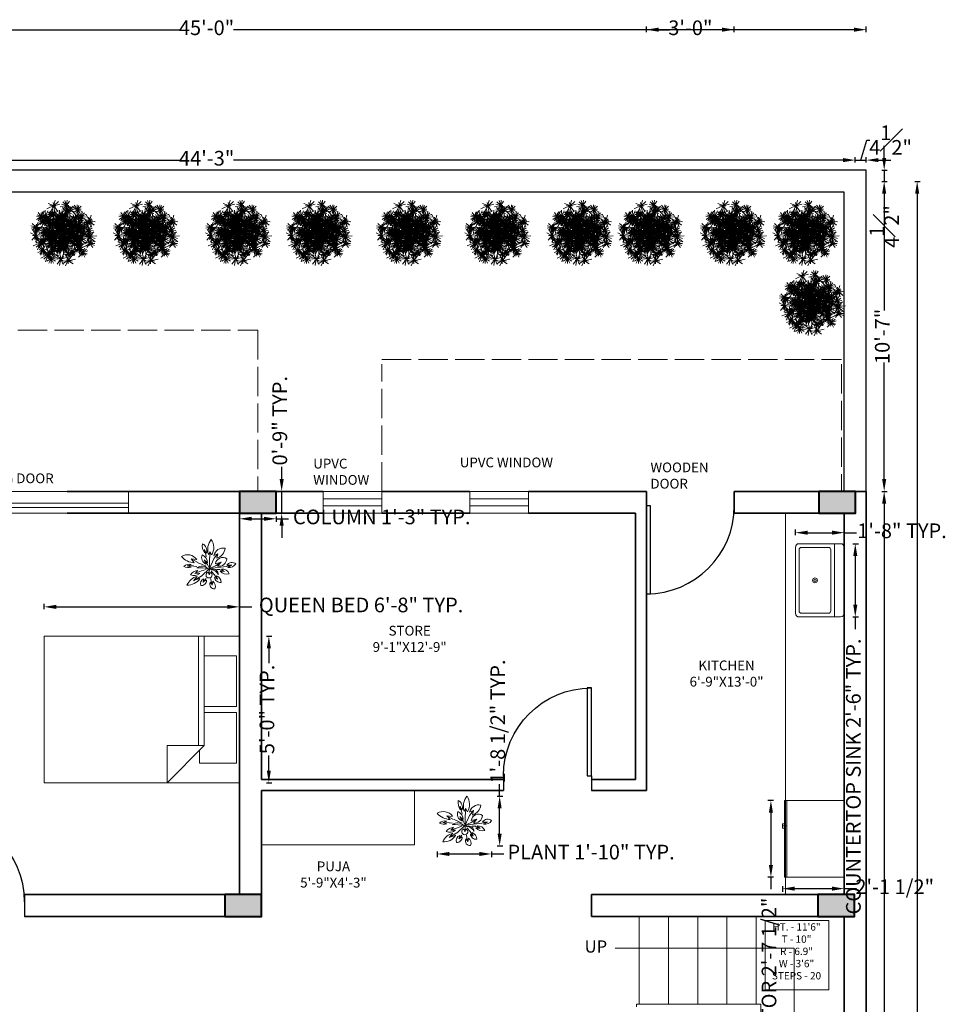
# Model space of a CAD drawing. Units: inches. Extents: x 2845 to 3575, y 808 to 1996.
# Tile 6 of 6: x 3166 to 3545, y 1588 to 1991. Entities that reach past the tile are written whole.
import ezdxf

# ---------------------------------------------------------------- set-up
doc = ezdxf.new("R2010")
doc.units = ezdxf.units.IN
doc.linetypes.add('ACAD_ISO02W100', pattern=[15, 12, -3])
for name, color, linetype, lineweight in [('A-ANNO-DIMS', 2, 'Continuous', 18), ('A-ANNO-SYMB', 7, 'Continuous', 18), ('A-ANNO-TEXT', 7, 'Continuous', 18), ('A-AREA-IDEN', 7, 'Continuous', 18), ('A-COLS', 7, 'Continuous', 40), ('A-DOOR', 34, 'Continuous', 25), ('A-EQPM', 8, 'Continuous', 18), ('A-FLOR-CASE', 30, 'Continuous', 18), ('A-FLOR-FIXT', 8, 'Continuous', 18), ('A-FLOR-STRS', 142, 'Continuous', 18), ('A-FURN', 30, 'Continuous', 18), ('A-GLAZ', 4, 'Continuous', 18), ('A-ROOF-OVHD', 7, 'ACAD_ISO02W100', 18), ('A-WALL', 1, 'Continuous', 35), ('C-PROP', 7, 'Continuous', 30), ('L-PLNT', 3, 'Continuous', 13)]:
    doc.layers.add(name, color=color, linetype=linetype, lineweight=lineweight)
doc.styles.get("Standard").update_dxf_attribs({"font": 'arial.ttf'})
doc.dimstyles.new('ISO-25', dxfattribs={"dimtxt": 6, "dimasz": 5, "dimexe": 1.25, "dimexo": 0.625, "dimtad": 0, "dimlunit": 4, "dimtxsty": 'Standard', "dimcen": 2.5, "dimclrd": 1, "dimclre": 1, "dimclrt": 1, "dimadec": 0, "dimazin": 0, "dimtfac": 1, "dimtmove": 0, "dimatfit": 3, "dimfxl": 1, "dimfxlon": 1, "dimfrac": 1, "dimarcsym": 0})

# ---------------------------------------------------------------- blocks, each defined once
blk = doc.blocks.new('*U3')
for p, q in [((0, 0), (0, -6)), ((36, 0), (36, -6))]:
    blk.add_line(p, q)
blk.add_lwpolyline([(0, 0), (0, 36), (1.75, 36), (1.75, 0)], close=True)
blk.add_arc((0, 0), 36, 0, 90)
blk = doc.blocks.new('*U7')
for p, q in [((0, 0), (0, 6)), ((36, 0), (36, 6))]:
    blk.add_line(p, q)
blk.add_lwpolyline([(0, 0), (0, -36), (1.75, -36), (1.75, 0)], close=True)
blk.add_arc((0, 0), 36, 270, 0)
blk = doc.blocks.new('Bed - Queen')
for p, q in [((0, -80.00003), (0, 0)), ((0, 0), (59.99999, 0)), ((59.99999, 0), (59.99999, -80.00003)), ((7.99999, -1.2), (28.79998, -1.2)), ((7.99999, -14.4), (7.99999, -1.2)), ((28.79998, -1.2), (28.79998, -14.4)), ((31.19999, -1.2), (51.99999, -1.2)), ((31.19999, -14.4), (31.19999, -1.2)), ((51.99999, -1.2), (51.99999, -16.4)), ((0, -14.4), (44.8, -14.4)), ((59.99999, -29.6), (44.8, -14.4)), ((44.8, -14.4), (44.8, -29.6)), ((44.8, -16.8), (0, -16.8)), ((51.99999, -16.4), (46.79936, -16.4)), ((44.8, -29.6), (59.99999, -29.6)), ((59.99999, -80.00003), (0, -80.00003))]:
    blk.add_line(p, q)
blk = doc.blocks.new('Sink-single - 30 in top')
blk.add_line((-15, -3.999996), (15, -3.999996))
for points in [[(-13.5, 0), (13.5, 0)], [(-15, -18.499996), (-15, -1.5)], [(15, -1.5), (15, -18.499996)], [(-13.5, -17.499996), (-13.5, -6.499996)], [(-12.5, -5.499996), (12.5, -5.499996)], [(13.5, -6.499996), (13.5, -17.499996)], [(13.5, -19.999996), (-13.5, -19.999996)], [(12.5, -18.499996), (-12.5, -18.499996)]]:
    blk.add_lwpolyline(points)
for radius in [1, 0.5]:
    blk.add_circle((0, -11.999996), radius)
for centre, radius, start, end in [((-13.5, -1.5), 1.5, 90, 180), ((13.5, -1.5), 1.5, 0, 90), ((-12.5, -6.499996), 1, 90, 180), ((12.5, -6.499996), 1, 0, 90), ((-13.5, -18.499996), 1.5, 180, 270), ((-12.5, -17.499996), 1, 180, 270), ((12.5, -17.499996), 1, 270, 0), ((13.5, -18.499996), 1.5, 270, 0)]:
    blk.add_arc(centre, radius, start, end)
blk = doc.blocks.new('Refrigerator-2 door - 36 in top')
for p, q in [((0, -26.999999), (36, -26.999999)), ((12, -26.999999), (12, -28.999999)), ((11, -27.999999), (11, -28.999999)), ((11, -28.999999), (13, -28.999999)), ((13, -28.999999), (13, -27.999999))]:
    blk.add_line(p, q)
blk.add_lwpolyline([(0, -27.999999), (0, 0), (36, 0), (36, -27.999999)], close=True)
blk = doc.blocks.new('z_96')
for p, q in [((-282, 143), (-440, 264)), ((-279, 140), (-327, 271)), ((-280, 150), (-254, 304)), ((-277, 144), (-209, 319)), ((2, 182), (-93, 262)), ((-2, 184), (-55, 292)), ((1, 182), (29, 300)), ((4, 189), (59, 265)), ((6, 185), (92, 285)), ((-283, 139), (-471, 115)), ((-292, 134), (-431, 180)), ((-279, 142), (-398, 17)), ((-286, 137), (-375, 92)), ((-278, 140), (-313, -1)), ((-279, 135), (-307, 100)), ((-280, 150), (-304, 174)), ((-278, 131), (-222, 40)), ((-277, 137), (-129, 19)), ((-276, 141), (-147, 221)), ((-18, -6), (-275, 142)), ((-263, 140), (-131, 114)), ((-260, 142), (-98, 156)), ((-10, 183), (-130, 223)), ((-75, -25), (-112, 38)), ((-6, 186), (-100, 114)), ((-5, 182), (-87, 72)), ((-72, -35), (-42, 65)), ((-5, -3), (1, 176)), ((-1, 185), (126, 194)), ((0, 0), (389, 84)), ((2, 183), (70, 78)), ((10, 182), (88, 115)), ((164, -90), (143, 12)), ((163, -89), (239, 8)), ((393, 90), (274, 50)), ((393, 90), (285, 153)), ((393, 90), (294, 12)), ((393, 90), (354, 209)), ((391, 83), (363, 42)), ((393, 90), (479, 182)), ((393, 90), (515, 124)), ((393, 90), (494, 13)), ((393, 90), (517, 64)), ((393, 90), (443, -26)), ((396, 95), (439, 246)), ((409, 93), (456, 89)), ((-237, -199), (-392, -169)), ((-242, -196), (-391, -241)), ((-242, -199), (-330, -310)), ((-246, -194), (-283, -164)), ((-237, -199), (-267, -22)), ((-241, -202), (-259, -277)), ((-242, -202), (-48, -207)), ((-10, -6), (-236, -205)), ((-236, -201), (-139, -307)), ((-234, -202), (-196, -41)), ((-231, -196), (-205, -162)), ((-231, -206), (-147, -236)), ((-75, -39), (-157, -75)), ((-74, -33), (-152, -41)), ((-65, -33), (-136, -11)), ((-76, -36), (-103, -106)), ((-80, -29), (-90, -20)), ((-16, -6), (-75, -37)), ((-73, -35), (-72, -112)), ((-70, -40), (-38, -103)), ((-70, -41), (4, -57)), ((-68, -28), (-56, -19)), ((-5, -19), (164, -92)), ((167, -95), (37, -175)), ((161, -92), (74, -95)), ((159, -86), (86, -29)), ((164, -102), (119, -171)), ((163, -86), (138, -56)), ((164, -93), (157, -141)), ((160, -93), (268, -148)), ((164, -92), (234, -170)), ((165, -92), (296, -74)), ((167, -88), (276, -25)), ((167, -91), (187, -100)), ((167, -104), (188, -213)), ((168, -88), (194, -72))]:
    blk.add_line(p, q)
blk = doc.blocks.new('сосна 1')
for p, rotation in [((318, 388), 121.1570021628385), ((-413, 387), 205.4822314301707), ((-343, -102), 57.88453704712605), ((-351, 122), 257.3134436407499), ((-143, -5), 121.1570021628385), ((-137, 361), 177.7388340989747), ((-117, 122), 55.05972244949475), ((286, 9), 60.73020616460848), ((234, -65), 73.8676290404427), ((-274, 161), 177.7388340989747), ((98, -5), 177.7388340989747), ((174, 17), 349.7944254651076), ((327, 46), 177.7388340989747), ((-502, -282), 279.7984529833926), ((-175, -367), 63.19571700542104), ((-49, -394), 342.5348703671633), ((261, -459), 13.72293452966709)]:
    blk.add_blockref('z_96', p, dxfattribs=dict(rotation=rotation))
blk = doc.blocks.new('z_109')
for p, q in [((-392, 202), (-278, 190)), ((-254, 128), (-392, 202)), ((-390, 202), (-327, 125)), ((-94, 294), (-122, 396)), ((-121, 393), (-119, 324)), ((-120, 377), (-82, 322)), ((-85, 244), (-94, 293)), ((-5, 350), (-42, 295)), ((-20, 11), (-18, 230)), ((-20, 11), (65, 205)), ((-14, 234), (-5, 350)), ((-5, 350), (24, 284)), ((65, 209), (150, 307)), ((65, 205), (65, 205)), ((150, 307), (68, 272)), ((129, 216), (150, 307)), ((150, 307), (129, 216)), ((-342, 60), (-472, 63)), ((-467, 63), (-392, 90)), ((-463, 64), (-392, 37)), ((-276, 53), (-338, 57)), ((-84, 54), (-246, 125)), ((-20, 11), (-181, -143)), ((-61, 92), (-128, 186)), ((-126, 184), (-60, 125)), ((-120, 176), (-91, 98)), ((-20, 11), (-61, 92)), ((-20, 11), (-24, -65)), ((-20, 11), (102, 64)), ((-20, 11), (-14, 11)), ((-14, 11), (319, 50)), ((-14, 11), (-13, 13)), ((-13, 13), (13, -13)), ((217, 135), (101, 105)), ((102, 64), (217, 135)), ((217, 135), (145, 55)), ((319, 50), (434, 75)), ((429, 74), (333, 77)), ((428, 74), (353, 32)), ((-187, -143), (-345, -240)), ((-342, -238), (-269, -151)), ((-328, -230), (-213, -195)), ((-178, -41), (-313, -92)), ((-308, -90), (-254, -33)), ((-306, -89), (-217, -88)), ((-86, -8), (-178, -41)), ((-89, -192), (-150, -267)), ((-150, -266), (-131, -199)), ((-26, -113), (-45, -66)), ((-24, -65), (-28, -121)), ((-28, -117), (-2, -69)), ((4, -192), (16, -238)), ((16, -43), (88, -126)), ((141, -208), (84, -170)), ((87, -129), (140, -204)), ((122, -8), (193, -11)), ((140, -205), (123, -139)), ((176, -10), (285, -54)), ((283, -54), (196, -42)), ((273, -52), (222, -4)), ((-151, -267), (-81, -228)), ((34, -320), (-6, -268)), ((16, -238), (35, -326)), ((35, -327), (45, -249))]:
    blk.add_line(p, q)
for centre, radius, start, end in [((84, 468), 249, 170.3029, 215.3262), ((-235, 368), 160, 343.2534, 62.5239), ((262, 393), 319, 140.563, 197.8988), ((-221, 433), 288, 328.6458, 34.5329), ((256, 231), 192, 77.7318, 167.6805), ((55, 447), 242, 287.7269, 353.3689), ((-464, 59), 228, 35.1725, 122.5976), ((-304, 504), 380, 221.8384, 266.6027), ((-21, 239), 158, 161.4501, 243.415), ((-251, 115), 192, 2.9136, 65.0019), ((247, 86), 147, 55.2824, 172.6291), ((167, 217), 164, 262.2896, 356.2544), ((-434, -39), 136, 71.6414, 139.5892), ((-450, 225), 197, 243.5199, 287.2599), ((-173, -118), 175, 44.3837, 127.1057), ((-243, -1063), 1086, 79.6239, 91.8656), ((434, 8), 123, 51.1111, 145.9654), ((384, 175), 146, 257.8549, 330.7421), ((-198, -444), 302, 103.499, 156.8265), ((-455, -39), 287, 265.8156, 327.2626), ((-246, -222), 190, 92.4489, 147.0817), ((-337, 52), 185, 248.0932, 310.529), ((-94, -301), 109, 109.8936, 199.3062), ((-31, -123), 58.9, 103.4106, 268.148), ((-26, -123), 58.9, 262.5922, 66.6581), ((53, -110), 105, 354.7987, 111.9005), ((2, -181), 167, 21.6922, 85.2277), ((197, -160), 113, 185.1842, 278.9266), ((66, -276), 148, 1.4924, 67.3596), ((325, 60), 164, 218.6232, 288.4099), ((241, -149), 146, 21.4559, 97.3107), ((-186, -232), 105, 264.4232, 2.0221), ((80, -308), 95.1, 155.1092, 275.9038), ((-28, -354), 128, 337.3115, 55.0978)]:
    blk.add_arc(centre, radius, start, end)
blk = doc.blocks.new('*D23')
at = {"layer": 'A-ANNO-DIMS', "color": 0, "lineweight": -2, "transparency": 16777216}
for p, q in [((2977.22, 1932.77), (2977.22, 1935.02)), ((3508.12, 1932.77), (3508.12, 1935.02)), ((2982.22, 1933.77), (3231.61, 1933.77)), ((3503.12, 1933.77), (3253.72, 1933.77))]:
    blk.add_line(p, q, dxfattribs=at)
at = {"layer": 'A-ANNO-DIMS', "color": 0, "transparency": 16777216}
for points in [[(2982.22, 1934.61), (2982.22, 1932.94), (2977.22, 1933.77)], [(3503.12, 1934.61), (3503.12, 1932.94), (3508.12, 1933.77)]]:
    blk.add_solid(points, dxfattribs=at)
at = {"layer": 'Defpoints', "color": 0, "transparency": 16777216}
for p in [(3508.12, 1933.77), (2977.22, 1929.67), (3508.12, 1920.75)]:
    blk.add_point(p, dxfattribs=at)
at = {"layer": 'A-ANNO-DIMS', "color": 0, "transparency": 16777216, "insert": (3242.67, 1933.77), "char_height": 6, "attachment_point": 5}
blk.add_mtext('44\'-3"', dxfattribs=at)
blk = doc.blocks.new('*D24')
at = {"layer": 'A-ANNO-DIMS', "color": 0, "lineweight": -2, "transparency": 16777216}
for p, q in [((3510.37, 1933.77), (3512.83, 1941.99)), ((3512.83, 1941.99), (3514.08, 1941.99)), ((3508.12, 1932.77), (3508.12, 1935.02)), ((3512.62, 1932.77), (3512.62, 1935.02)), ((3503.12, 1933.77), (3498.12, 1933.77)), ((3508.12, 1933.77), (3512.62, 1933.77)), ((3508.12, 1933.77), (3512.62, 1933.77)), ((3517.62, 1933.77), (3522.62, 1933.77))]:
    blk.add_line(p, q, dxfattribs=at)
at = {"layer": 'A-ANNO-DIMS', "color": 0, "transparency": 16777216}
for points in [[(3503.12, 1934.61), (3503.12, 1932.94), (3508.12, 1933.77)], [(3517.62, 1934.61), (3517.62, 1932.94), (3512.62, 1933.77)]]:
    blk.add_solid(points, dxfattribs=at)
at = {"layer": 'Defpoints', "color": 0, "transparency": 16777216}
for p in [(3512.62, 1933.77), (3512.62, 1929.67), (3508.12, 1920.75)]:
    blk.add_point(p, dxfattribs=at)
at = {"layer": 'A-ANNO-DIMS', "color": 0, "transparency": 16777216, "insert": (3522.57, 1941.99), "char_height": 6, "attachment_point": 5}
blk.add_mtext('4{\\H1x;\\S1#2;}"', dxfattribs=at)
blk = doc.blocks.new('*D25')
at = {"layer": 'A-ANNO-DIMS', "color": 0, "lineweight": -2, "transparency": 16777216}
for p, q in [((3519.95, 1934.67), (3519.95, 1939.67)), ((3518.95, 1929.67), (3521.2, 1929.67)), ((3519.95, 1929.67), (3519.95, 1925.07)), ((3518.95, 1925.07), (3521.2, 1925.07)), ((3519.95, 1920.07), (3519.95, 1915.07))]:
    blk.add_line(p, q, dxfattribs=at)
at = {"layer": 'A-ANNO-DIMS', "color": 0, "transparency": 16777216}
for points in [[(3519.11, 1934.67), (3520.78, 1934.67), (3519.95, 1929.67)], [(3519.11, 1920.07), (3520.78, 1920.07), (3519.95, 1925.07)]]:
    blk.add_solid(points, dxfattribs=at)
at = {"layer": 'Defpoints', "color": 0, "transparency": 16777216}
for p in [(3512.62, 1929.67), (3512.62, 1925.07), (3519.95, 1925.07)]:
    blk.add_point(p, dxfattribs=at)
at = {"layer": 'A-ANNO-DIMS', "color": 0, "transparency": 16777216, "insert": (3519.95, 1906.59), "char_height": 6, "attachment_point": 5, "rotation": 90}
blk.add_mtext('4{\\H1x;\\S1#2;}"', dxfattribs=at)
blk = doc.blocks.new('*D26')
at = {"layer": 'A-ANNO-DIMS', "color": 0, "lineweight": -2, "transparency": 16777216}
for p, q in [((3518.95, 1925.07), (3521.2, 1925.07)), ((3519.95, 1920.07), (3519.95, 1872.27)), ((3519.95, 1803.17), (3519.95, 1850.97)), ((3518.95, 1798.17), (3521.2, 1798.17))]:
    blk.add_line(p, q, dxfattribs=at)
at = {"layer": 'A-ANNO-DIMS', "color": 0, "transparency": 16777216}
for points in [[(3519.11, 1920.07), (3520.78, 1920.07), (3519.95, 1925.07)], [(3519.11, 1803.17), (3520.78, 1803.17), (3519.95, 1798.17)]]:
    blk.add_solid(points, dxfattribs=at)
at = {"layer": 'Defpoints', "color": 0, "transparency": 16777216}
for p in [(3512.62, 1925.07), (3512.62, 1798.17), (3519.95, 1798.17)]:
    blk.add_point(p, dxfattribs=at)
at = {"layer": 'A-ANNO-DIMS', "color": 0, "transparency": 16777216, "insert": (3519.95, 1861.62), "char_height": 6, "attachment_point": 5, "rotation": 90}
blk.add_mtext('10\'-7"', dxfattribs=at)
blk = doc.blocks.new('*D27')
at = {"layer": 'A-ANNO-DIMS', "color": 0, "lineweight": -2, "transparency": 16777216}
for p, q in [((3518.95, 1798.17), (3521.2, 1798.17)), ((3519.95, 1793.17), (3519.95, 1512.51)), ((3519.95, 1220.17), (3519.95, 1500.84)), ((3518.95, 1215.17), (3521.2, 1215.17))]:
    blk.add_line(p, q, dxfattribs=at)
at = {"layer": 'A-ANNO-DIMS', "color": 0, "transparency": 16777216}
for points in [[(3519.11, 1793.17), (3520.78, 1793.17), (3519.95, 1798.17)], [(3519.11, 1220.17), (3520.78, 1220.17), (3519.95, 1215.17)]]:
    blk.add_solid(points, dxfattribs=at)
at = {"layer": 'Defpoints', "color": 0, "transparency": 16777216}
for p in [(3512.62, 1798.17), (3507.65, 1215.17), (3519.95, 1215.17)]:
    blk.add_point(p, dxfattribs=at)
at = {"layer": 'A-ANNO-DIMS', "color": 0, "transparency": 16777216, "insert": (3519.95, 1506.67), "char_height": 6, "attachment_point": 5, "rotation": 90}
blk.add_mtext("49'", dxfattribs=at)
blk = doc.blocks.new('*D29')
at = {"layer": 'A-ANNO-DIMS', "color": 0, "lineweight": -2, "transparency": 16777216}
for p, q in [((3532.44, 1925.07), (3534.69, 1925.07)), ((3533.44, 1920.07), (3533.44, 1464.53)), ((3533.44, 987.17), (3533.44, 1442.72)), ((3532.44, 982.17), (3534.69, 982.17))]:
    blk.add_line(p, q, dxfattribs=at)
at = {"layer": 'A-ANNO-DIMS', "color": 0, "transparency": 16777216}
for points in [[(3532.6, 1920.07), (3534.27, 1920.07), (3533.44, 1925.07)], [(3532.6, 987.17), (3534.27, 987.17), (3533.44, 982.17)]]:
    blk.add_solid(points, dxfattribs=at)
at = {"layer": 'Defpoints', "color": 0, "transparency": 16777216}
for p in [(3519.95, 1925.07), (3533.44, 1925.07), (3512.62, 982.17)]:
    blk.add_point(p, dxfattribs=at)
at = {"layer": 'A-ANNO-DIMS', "color": 0, "transparency": 16777216, "insert": (3533.44, 1453.62), "char_height": 6, "attachment_point": 5, "rotation": 90}
blk.add_mtext('78\'-7"', dxfattribs=at)
blk = doc.blocks.new('COL-15x9')
h = blk.add_hatch(color=256)
h.dxf.hatch_style = 1
h.paths.add_polyline_path([(15, 9), (0, 9), (0, 0), (15, 0)])
blk.add_lwpolyline([(0, 9), (0, 0), (15, 0), (15, 9)], close=True)
blk = doc.blocks.new('WIN-24')
for p, q in [((0, 9), (0, 0)), ((0, 9), (24, 9)), ((24, 9), (24, 0)), ((0, 6), (24, 6)), ((0, 3), (24, 3)), ((0, 0), (24, 0))]:
    blk.add_line(p, q)
blk = doc.blocks.new('GLAZ-SLIDER-97')
for p, q in [((0, 9), (0, 0)), ((0, 9), (97.12, 9)), ((97.12, 9), (97.12, 0)), ((0, 6.63), (48.56, 6.63)), ((48.56, 4.89), (0, 4.89)), ((48.56, 6.63), (48.56, 4.89)), ((48.56, 2.45), (48.56, 4.19)), ((48.56, 4.19), (97.12, 4.19)), ((0, 0), (97.12, 0)), ((97.12, 2.45), (48.56, 2.45))]:
    blk.add_line(p, q)
blk = doc.blocks.new('*D40')
at = {"layer": 'A-ANNO-DIMS', "color": 1, "lineweight": -2, "transparency": 16777216}
for p, q in [((3337.01, 1650.72), (3337.01, 1648.47)), ((3342.01, 1649.72), (3354.24, 1649.72)), ((3359.24, 1650.72), (3359.24, 1648.47)), ((3359.24, 1649.72), (3364.24, 1649.72))]:
    blk.add_line(p, q, dxfattribs=at)
at = {"layer": 'A-ANNO-DIMS', "color": 1, "transparency": 16777216}
for points in [[(3342.01, 1650.55), (3342.01, 1648.89), (3337.01, 1649.72)], [(3354.24, 1650.55), (3354.24, 1648.89), (3359.24, 1649.72)]]:
    blk.add_solid(points, dxfattribs=at)
at = {"layer": 'Defpoints', "color": 0, "transparency": 16777216}
for p in [(3337.01, 1653.05), (3359.24, 1653.05), (3359.24, 1649.72)]:
    blk.add_point(p, dxfattribs=at)
at = {"layer": 'A-ANNO-DIMS', "color": 1, "transparency": 16777216, "insert": (3400, 1649.72), "char_height": 6, "attachment_point": 5}
blk.add_mtext('PLANT 1\'-10" TYP.', dxfattribs=at)
blk = doc.blocks.new('*D41')
at = {"layer": 'A-ANNO-DIMS', "color": 1, "lineweight": -2, "transparency": 16777216}
for p, q in [((3362.57, 1673.34), (3362.57, 1678.34)), ((3361.57, 1673.34), (3363.82, 1673.34)), ((3362.57, 1658.05), (3362.57, 1668.34)), ((3361.57, 1653.05), (3363.82, 1653.05))]:
    blk.add_line(p, q, dxfattribs=at)
at = {"layer": 'A-ANNO-DIMS', "color": 1, "transparency": 16777216}
for points in [[(3361.74, 1668.34), (3363.4, 1668.34), (3362.57, 1673.34)], [(3361.74, 1658.05), (3363.4, 1658.05), (3362.57, 1653.05)]]:
    blk.add_solid(points, dxfattribs=at)
at = {"layer": 'Defpoints', "color": 0, "transparency": 16777216}
for p in [(3359.24, 1673.34), (3362.57, 1673.34), (3359.24, 1653.05)]:
    blk.add_point(p, dxfattribs=at)
at = {"layer": 'A-ANNO-DIMS', "color": 1, "transparency": 16777216, "insert": (3362.57, 1703.96), "char_height": 6, "attachment_point": 5, "rotation": 90}
blk.add_mtext('1\'-8 1/2" TYP.', dxfattribs=at)
blk = doc.blocks.new('*D42')
at = {"layer": 'A-ANNO-DIMS', "color": 1, "lineweight": -2, "transparency": 16777216}
for p, q in [((3256.12, 1787.92), (3256.12, 1785.67)), ((3261.12, 1786.92), (3266.12, 1786.92)), ((3271.12, 1787.92), (3271.12, 1785.67)), ((3271.12, 1786.92), (3276.12, 1786.92))]:
    blk.add_line(p, q, dxfattribs=at)
at = {"layer": 'A-ANNO-DIMS', "color": 1, "transparency": 16777216}
for points in [[(3261.12, 1787.76), (3261.12, 1786.09), (3256.12, 1786.92)], [(3266.12, 1787.76), (3266.12, 1786.09), (3271.12, 1786.92)]]:
    blk.add_solid(points, dxfattribs=at)
at = {"layer": 'Defpoints', "color": 0, "transparency": 16777216}
for p in [(3256.12, 1789.17), (3271.12, 1789.17), (3271.12, 1786.92)]:
    blk.add_point(p, dxfattribs=at)
at = {"layer": 'A-ANNO-DIMS', "color": 1, "transparency": 16777216, "insert": (3314.32, 1786.92), "char_height": 6, "attachment_point": 5}
blk.add_mtext('COLUMN 1\'-3" TYP.', dxfattribs=at)
blk = doc.blocks.new('*D43')
at = {"layer": 'A-ANNO-DIMS', "color": 1, "lineweight": -2, "transparency": 16777216}
for p, q in [((3273.37, 1803.17), (3273.37, 1808.17)), ((3272.37, 1798.17), (3274.62, 1798.17)), ((3273.37, 1789.17), (3273.37, 1798.17)), ((3272.37, 1789.17), (3274.62, 1789.17)), ((3273.37, 1784.17), (3273.37, 1779.17))]:
    blk.add_line(p, q, dxfattribs=at)
at = {"layer": 'A-ANNO-DIMS', "color": 1, "transparency": 16777216}
for points in [[(3272.53, 1803.17), (3274.2, 1803.17), (3273.37, 1798.17)], [(3272.53, 1784.17), (3274.2, 1784.17), (3273.37, 1789.17)]]:
    blk.add_solid(points, dxfattribs=at)
at = {"layer": 'Defpoints', "color": 0, "transparency": 16777216}
for p in [(3271.12, 1798.17), (3273.37, 1798.17), (3271.12, 1789.17)]:
    blk.add_point(p, dxfattribs=at)
at = {"layer": 'A-ANNO-DIMS', "color": 1, "transparency": 16777216, "insert": (3273.37, 1827.08), "char_height": 6, "attachment_point": 5, "rotation": 90}
blk.add_mtext('0\'-9" TYP.', dxfattribs=at)
blk = doc.blocks.new('*D48')
at = {"layer": 'A-ANNO-DIMS', "color": 1, "lineweight": -2, "transparency": 16777216}
for p, q in [((3507.12, 1776.75), (3509.37, 1776.75)), ((3508.12, 1771.75), (3508.12, 1751.75)), ((3507.12, 1746.75), (3509.37, 1746.75)), ((3508.12, 1746.75), (3508.12, 1741.75))]:
    blk.add_line(p, q, dxfattribs=at)
at = {"layer": 'A-ANNO-DIMS', "color": 1, "transparency": 16777216}
for points in [[(3507.28, 1771.75), (3508.95, 1771.75), (3508.12, 1776.75)], [(3507.28, 1751.75), (3508.95, 1751.75), (3508.12, 1746.75)]]:
    blk.add_solid(points, dxfattribs=at)
at = {"layer": 'Defpoints', "color": 0, "transparency": 16777216}
for p in [(3503.62, 1776.75), (3503.62, 1746.75), (3508.12, 1746.75)]:
    blk.add_point(p, dxfattribs=at)
at = {"layer": 'A-ANNO-DIMS', "color": 1, "transparency": 16777216, "insert": (3508.12, 1681.43), "char_height": 6, "attachment_point": 5, "rotation": 90}
blk.add_mtext('COUNTERTOP SINK 2\'-6" TYP.', dxfattribs=at)
blk = doc.blocks.new('*D49')
at = {"layer": 'A-ANNO-DIMS', "color": 1, "lineweight": -2, "transparency": 16777216}
for p, q in [((3483.62, 1780.25), (3483.62, 1782.5)), ((3503.62, 1780.25), (3503.62, 1782.5)), ((3488.62, 1781.25), (3498.62, 1781.25)), ((3503.62, 1781.25), (3508.62, 1781.25))]:
    blk.add_line(p, q, dxfattribs=at)
at = {"layer": 'A-ANNO-DIMS', "color": 1, "transparency": 16777216}
for points in [[(3488.62, 1782.08), (3488.62, 1780.42), (3483.62, 1781.25)], [(3498.62, 1782.08), (3498.62, 1780.42), (3503.62, 1781.25)]]:
    blk.add_solid(points, dxfattribs=at)
at = {"layer": 'Defpoints', "color": 0, "transparency": 16777216}
for p in [(3503.62, 1781.25), (3483.62, 1776.75), (3503.62, 1776.75)]:
    blk.add_point(p, dxfattribs=at)
at = {"layer": 'A-ANNO-DIMS', "color": 1, "transparency": 16777216, "insert": (3527.24, 1781.25), "char_height": 6, "attachment_point": 5}
blk.add_mtext('1\'-8" TYP.', dxfattribs=at)
blk = doc.blocks.new('*D50')
at = {"layer": 'A-ANNO-DIMS', "color": 1, "lineweight": -2, "transparency": 16777216}
for p, q in [((3176.12, 1749.88), (3176.12, 1752.13)), ((3181.12, 1750.88), (3251.12, 1750.88)), ((3256.12, 1749.88), (3256.12, 1752.13)), ((3256.12, 1750.88), (3261.12, 1750.88))]:
    blk.add_line(p, q, dxfattribs=at)
at = {"layer": 'A-ANNO-DIMS', "color": 1, "transparency": 16777216}
for points in [[(3181.12, 1751.71), (3181.12, 1750.04), (3176.12, 1750.88)], [(3251.12, 1751.71), (3251.12, 1750.04), (3256.12, 1750.88)]]:
    blk.add_solid(points, dxfattribs=at)
at = {"layer": 'Defpoints', "color": 0, "transparency": 16777216}
for p in [(3256.12, 1750.88), (3176.12, 1738.88), (3256.12, 1738.88)]:
    blk.add_point(p, dxfattribs=at)
at = {"layer": 'A-ANNO-DIMS', "color": 1, "transparency": 16777216, "insert": (3305.87, 1750.88), "char_height": 6, "attachment_point": 5}
blk.add_mtext('QUEEN BED 6\'-8" TYP.', dxfattribs=at)
blk = doc.blocks.new('*D51')
at = {"layer": 'A-ANNO-DIMS', "color": 1, "lineweight": -2, "transparency": 16777216}
for p, q in [((3267.12, 1738.88), (3269.37, 1738.88)), ((3268.12, 1733.88), (3268.12, 1727.79)), ((3268.12, 1683.88), (3268.12, 1689.97)), ((3267.12, 1678.88), (3269.37, 1678.88))]:
    blk.add_line(p, q, dxfattribs=at)
at = {"layer": 'A-ANNO-DIMS', "color": 1, "transparency": 16777216}
for points in [[(3267.28, 1733.88), (3268.95, 1733.88), (3268.12, 1738.88)], [(3267.28, 1683.88), (3268.95, 1683.88), (3268.12, 1678.88)]]:
    blk.add_solid(points, dxfattribs=at)
at = {"layer": 'Defpoints', "color": 0, "transparency": 16777216}
for p in [(3256.12, 1738.88), (3256.12, 1678.88), (3268.12, 1678.88)]:
    blk.add_point(p, dxfattribs=at)
at = {"layer": 'A-ANNO-DIMS', "color": 1, "transparency": 16777216, "insert": (3268.12, 1708.88), "char_height": 6, "attachment_point": 5, "rotation": 90}
blk.add_mtext('5\'-0" TYP.', dxfattribs=at)
blk = doc.blocks.new('*D68')
at = {"layer": 'A-ANNO-DIMS', "color": 1, "lineweight": -2, "transparency": 16777216}
for p, q in [((3474.59, 1671.66), (3472.34, 1671.66)), ((3473.59, 1666.66), (3473.59, 1645.24)), ((3474.59, 1640.24), (3472.34, 1640.24)), ((3473.59, 1640.24), (3473.59, 1635.24))]:
    blk.add_line(p, q, dxfattribs=at)
at = {"layer": 'A-ANNO-DIMS', "color": 1, "transparency": 16777216}
for points in [[(3472.76, 1666.66), (3474.42, 1666.66), (3473.59, 1671.66)], [(3472.76, 1645.24), (3474.42, 1645.24), (3473.59, 1640.24)]]:
    blk.add_solid(points, dxfattribs=at)
at = {"layer": 'Defpoints', "color": 0, "transparency": 16777216}
for p in [(3478.3, 1671.66), (3473.59, 1640.24), (3478.3, 1640.24)]:
    blk.add_point(p, dxfattribs=at)
at = {"layer": 'A-ANNO-DIMS', "color": 1, "transparency": 16777216, "insert": (3473.59, 1585.34), "char_height": 6, "attachment_point": 5, "rotation": 90}
blk.add_mtext('REFRIGERATOR 2\'-7 1/2"', dxfattribs=at)
blk = doc.blocks.new('*D69')
at = {"layer": 'A-ANNO-DIMS', "color": 1, "lineweight": -2, "transparency": 16777216}
for p, q in [((3478.3, 1636.52), (3478.3, 1634.27)), ((3483.3, 1635.52), (3498.62, 1635.52)), ((3503.62, 1636.52), (3503.62, 1634.27)), ((3503.62, 1635.52), (3508.62, 1635.52))]:
    blk.add_line(p, q, dxfattribs=at)
at = {"layer": 'A-ANNO-DIMS', "color": 1, "transparency": 16777216}
for points in [[(3483.3, 1636.36), (3483.3, 1634.69), (3478.3, 1635.52)], [(3498.62, 1636.36), (3498.62, 1634.69), (3503.62, 1635.52)]]:
    blk.add_solid(points, dxfattribs=at)
at = {"layer": 'Defpoints', "color": 0, "transparency": 16777216}
for p in [(3478.3, 1640.24), (3503.62, 1640.24), (3503.62, 1635.52)]:
    blk.add_point(p, dxfattribs=at)
at = {"layer": 'A-ANNO-DIMS', "color": 1, "transparency": 16777216, "insert": (3524.26, 1635.52), "char_height": 6, "attachment_point": 5}
blk.add_mtext('2\'-1 1/2"', dxfattribs=at)
blk = doc.blocks.new('*D70')
at = {"layer": 'A-ANNO-DIMS', "color": 1, "lineweight": -2, "transparency": 16777216}
for p, q in [((2972.62, 1986.17), (2972.62, 1988.42)), ((3512.62, 1986.17), (3512.62, 1988.42)), ((2977.62, 1987.17), (3231.56, 1987.17)), ((3507.62, 1987.17), (3253.67, 1987.17))]:
    blk.add_line(p, q, dxfattribs=at)
at = {"layer": 'A-ANNO-DIMS', "color": 1, "transparency": 16777216}
for points in [[(2977.62, 1988.01), (2977.62, 1986.34), (2972.62, 1987.17)], [(3507.62, 1988.01), (3507.62, 1986.34), (3512.62, 1987.17)]]:
    blk.add_solid(points, dxfattribs=at)
at = {"layer": 'Defpoints', "color": 0, "transparency": 16777216}
for p in [(3512.62, 1987.17), (2972.62, 1929.67), (3512.62, 1929.67)]:
    blk.add_point(p, dxfattribs=at)
at = {"layer": 'A-ANNO-DIMS', "color": 1, "transparency": 16777216, "insert": (3242.62, 1987.17), "char_height": 6, "attachment_point": 5}
blk.add_mtext('45\'-0"', dxfattribs=at)
blk = doc.blocks.new('*D75')
at = {"layer": 'A-ANNO-DIMS', "color": 1, "lineweight": -2, "transparency": 16777216}
for p, q in [((3422.62, 1986.17), (3422.62, 1988.42)), ((3458.62, 1986.17), (3458.62, 1988.42)), ((3427.62, 1987.17), (3432.02, 1987.17)), ((3453.62, 1987.17), (3449.21, 1987.17))]:
    blk.add_line(p, q, dxfattribs=at)
at = {"layer": 'A-ANNO-DIMS', "color": 1, "transparency": 16777216}
for points in [[(3427.62, 1988.01), (3427.62, 1986.34), (3422.62, 1987.17)], [(3453.62, 1988.01), (3453.62, 1986.34), (3458.62, 1987.17)]]:
    blk.add_solid(points, dxfattribs=at)
at = {"layer": 'Defpoints', "color": 0, "transparency": 16777216}
for p in [(3458.62, 1987.17), (3422.62, 1798.17), (3458.62, 1798.17)]:
    blk.add_point(p, dxfattribs=at)
at = {"layer": 'A-ANNO-DIMS', "color": 1, "transparency": 16777216, "insert": (3440.62, 1987.17), "char_height": 6, "attachment_point": 5}
blk.add_mtext('3\'-0"', dxfattribs=at)

msp = doc.modelspace()

# ---------------------------------------------------------------- linework, layer by layer
at = {"layer": 'A-ANNO-SYMB'}
for p, q in [((3409.905, 1611.198), (3483.127, 1611.198)), ((3483.127, 1611.198), (3483.127, 1544.532))]:
    msp.add_line(p, q, dxfattribs=at)
msp.add_lwpolyline([(3471.295, 1622.497), (3497.24, 1622.497), (3497.24, 1594.13), (3471.295, 1594.13)], close=True, dxfattribs=at)
at = {"layer": 'A-DOOR'}
for p, q in [((3458.616, 1798.173), (3458.616, 1789.173)), ((3364.116, 1680.173), (3364.116, 1675.673)), ((3400.116, 1680.173), (3400.116, 1675.673)), ((3168.116, 1633.173), (3168.116, 1624.173))]:
    msp.add_line(p, q, dxfattribs=at)
at = {"layer": 'A-FLOR-CASE'}
for p, q in [((3479.616, 1633.173), (3479.616, 1789.173)), ((3327.679, 1675.673), (3327.679, 1653.472)), ((3327.679, 1653.472), (3265.116, 1653.472))]:
    msp.add_line(p, q, dxfattribs=at)
at = {"layer": 'A-FLOR-STRS'}
for p, q in [((3419.616, 1588.173), (3419.616, 1624.173)), ((3431.616, 1588.173), (3431.616, 1624.173)), ((3443.616, 1588.173), (3443.616, 1624.173)), ((3455.616, 1588.173), (3455.616, 1624.173)), ((3467.616, 1588.173), (3467.616, 1624.173)), ((3418.616, 1587.173), (3418.616, 1588.173)), ((3418.616, 1588.173), (3419.616, 1588.173)), ((3419.616, 1588.173), (3469.473, 1588.173)), ((3469.473, 1588.173), (3469.473, 1527.173))]:
    msp.add_line(p, q, dxfattribs=at)
at = {"layer": 'A-ROOF-OVHD'}
for p, q in [((3075.459, 1864.202), (3263.616, 1864.202)), ((3263.616, 1864.202), (3263.616, 1798.173)), ((3314.316, 1852.202), (3502.472, 1852.202)), ((3314.316, 1798.173), (3314.316, 1850.202)), ((3502.472, 1850.202), (3502.472, 1798.173))]:
    msp.add_line(p, q, dxfattribs=at)
at = {"layer": 'A-WALL'}
for p, q in [((3290.316, 1798.173), (3185.616, 1798.173)), ((3256.116, 1789.173), (3256.116, 1798.173)), ((3271.116, 1798.173), (3271.116, 1789.173)), ((3350.316, 1798.173), (3314.316, 1798.173)), ((3422.616, 1798.173), (3374.316, 1798.173)), ((3422.616, 1675.673), (3422.616, 1798.173)), ((3503.616, 1798.173), (3458.616, 1798.173)), ((3503.616, 1798.173), (3512.616, 1798.173)), ((3512.616, 1159.066), (3512.616, 1798.173)), ((3265.116, 1789.173), (3185.616, 1789.173)), ((3256.116, 1633.173), (3256.116, 1789.173)), ((3265.116, 1680.173), (3265.116, 1789.173)), ((3290.316, 1789.173), (3265.116, 1789.173)), ((3350.316, 1789.173), (3314.316, 1789.173)), ((3418.116, 1789.173), (3374.316, 1789.173)), ((3418.116, 1680.173), (3418.116, 1789.173)), ((3503.616, 1789.173), (3458.616, 1789.173)), ((3503.616, 1633.173), (3503.616, 1789.173)), ((3364.116, 1680.173), (3265.116, 1680.173)), ((3418.116, 1680.173), (3400.116, 1680.173)), ((3265.116, 1624.173), (3265.116, 1675.673)), ((3364.116, 1675.673), (3265.116, 1675.673)), ((3422.616, 1675.673), (3400.116, 1675.673)), ((3265.116, 1633.173), (3168.116, 1633.173)), ((3400.116, 1624.173), (3400.116, 1633.173)), ((3265.116, 1624.173), (3168.116, 1624.173)), ((3503.616, 1450.173), (3503.616, 1624.173))]:
    msp.add_line(p, q, dxfattribs=at)
for points in [[(3400.116, 1633.173), (3418.116, 1633.173), (3503.616, 1633.173)], [(3503.616, 1624.173), (3418.116, 1624.173), (3400.116, 1624.173)]]:
    msp.add_lwpolyline(points, dxfattribs=at)
at = {"layer": 'C-PROP'}
for p, q in [((3512.616, 1929.673), (2972.616, 1929.673)), ((3512.616, 1798.173), (3512.616, 1929.673)), ((3503.616, 1920.673), (2981.616, 1920.673)), ((3503.616, 1798.173), (3503.616, 1920.673))]:
    msp.add_line(p, q, dxfattribs=at)

# ---------------------------------------------------------------- block references
at = {"layer": 'A-COLS'}
for p in [(3256.116, 1789.173), (3493.219, 1789.173), (3250.141, 1624.173), (3492.783, 1624.173)]:
    msp.add_blockref('COL-15x9', p, dxfattribs=at)
at = {"layer": 'A-DOOR'}
for name, p in [('*U7', (3422.616, 1792.173)), ('*U3', (3132.116, 1630.173))]:
    msp.add_blockref(name, p, dxfattribs=at)
at = {"layer": 'A-DOOR', "xscale": -1}
msp.add_blockref('*U3', (3400.116, 1681.673), dxfattribs=at)
at = {"layer": 'A-EQPM', "xscale": 0.8728317921311891, "yscale": 0.8728317921311891, "zscale": 0.8728317921311891, "rotation": 270}
msp.add_blockref('Refrigerator-2 door - 36 in top', (3503.616, 1671.658), dxfattribs=at)
at = {"layer": 'A-FLOR-FIXT', "rotation": 270}
msp.add_blockref('Sink-single - 30 in top', (3503.616, 1761.749), dxfattribs=at)
at = {"layer": 'A-FURN', "rotation": 270}
msp.add_blockref('Bed - Queen', (3256.116, 1738.877), dxfattribs=at)
at = {"layer": 'A-GLAZ'}
for name, p in [('GLAZ-SLIDER-97', (3113.616, 1789.173)), ('WIN-24', (3290.316, 1789.173)), ('WIN-24', (3350.316, 1789.173))]:
    msp.add_blockref(name, p, dxfattribs=at)
at = {"layer": 'L-PLNT'}
for name, p, xscale, yscale, zscale in [('сосна 1', (3184.722, 1904.174), 0.0163507860903289, 0.0163507860903289, 0.0163507860903289), ('сосна 1', (3218.523, 1904.174), 0.0163507860903289, 0.0163507860903289, 0.0163507860903289), ('сосна 1', (3256.314, 1904.174), 0.0163507860903289, 0.0163507860903289, 0.0163507860903289), ('сосна 1', (3289.299, 1904.174), 0.0163507860903289, 0.0163507860903289, 0.0163507860903289), ('сосна 1', (3326.164, 1904.174), 0.0163507860903289, 0.0163507860903289, 0.0163507860903289), ('сосна 1', (3362.383, 1904.174), 0.0163507860903289, 0.0163507860903289, 0.0163507860903289), ('сосна 1', (3396.015, 1904.174), 0.0163507860903289, 0.0163507860903289, 0.0163507860903289), ('сосна 1', (3425.119, 1904.174), 0.0163507860903289, 0.0163507860903289, 0.0163507860903289), ('сосна 1', (3458.751, 1904.174), 0.0163507860903289, 0.0163507860903289, 0.0163507860903289), ('сосна 1', (3488.502, 1904.174), 0.0163507860903289, 0.0163507860903289, 0.0163507860903289), ('сосна 1', (3491.089, 1875.49), 0.0163507860903289, 0.0163507860903289, 0.0163507860903289), ('z_109', (3244.226, 1766.396), 0.0202275909996564, 0.0202275909996564, 0.0202275909996564), ('z_109', (3348.889, 1661.276), 0.0202275909996564, 0.0202275909996564, 0.0202275909996564)]:
    msp.add_blockref(name, p, dxfattribs=dict(at, xscale=xscale, yscale=yscale, zscale=zscale))

# ---------------------------------------------------------------- texts
at = {"layer": 'A-ANNO-SYMB', "insert": (3397.345, 1614.327), "char_height": 5, "attachment_point": 1}
msp.add_mtext_dynamic_manual_height_columns('UP', width=32.32705, gutter_width=12.5, heights=[0], dxfattribs=at)
at = {"layer": 'A-ANNO-TEXT', "attachment_point": 1}
for s, width, insert, char_height in [('UPVC WINDOW', 27.40312, (3286.287, 1811.525), 4), ('UPVC WINDOW', 45.255, (3346.263, 1812.007), 4), ('WOODEN DOOR', 35.20843, (3424.288, 1809.977), 4), ('UPVC SLIDING DOOR', 60.26056, (3127.413, 1805.497), 4), ('\\pxqc;HT. - 11\'6"\\PT - 10"\\PR - 6.9"\\PW - 3\'6"\\PSTEPS - 20', 48.6981, (3459.726, 1621.354), 3)]:
    msp.add_mtext_dynamic_manual_height_columns(s, width=width, gutter_width=12.5, heights=[0], dxfattribs=dict(at, insert=insert, char_height=char_height))
at = {"layer": 'A-AREA-IDEN', "char_height": 4, "attachment_point": 1}
for s, heights, insert in [('\\pxqc;STORE\\P9\'-1"X12\'-9"', [0], (3303.128, 1743.124)), ('\\pxqc;KITCHEN\\P6\'-9"X13\'-0"', [13.021], (3432.809, 1728.914)), ('\\pxqc;PUJA\\P5\'-9"X4\'-3"', [0], (3271.935, 1646.654))]:
    msp.add_mtext_dynamic_manual_height_columns(s, width=45.255, gutter_width=12.5, heights=heights, dxfattribs=dict(at, insert=insert))

# ---------------------------------------------------------------- dimensions: what is measured, and where the dimension line sits
at = {"layer": 'A-ANNO-DIMS'}
for base, p1, p2, override, picture, middle in [((3512.616, 1987.173), (2972.616, 1929.673), (3512.616, 1929.673), {"dimdec": 1, "dimlfac": 1, "dimrnd": 0, "dimzin": 1, "dimdsep": 46, "dimlunit": 4, "dimfrac": 2}, '*D70', (3242.616, 1987.173)), ((3458.616, 1987.173), (3422.616, 1798.173), (3458.616, 1798.173), {"dimdec": 1, "dimlfac": 1, "dimrnd": 0, "dimzin": 1, "dimdsep": 46, "dimlunit": 4, "dimfrac": 2}, '*D75', (3440.616, 1987.173)), ((3512.616, 1933.775), (3508.116, 1920.754), (3512.616, 1929.673), {"dimclrd": 0, "dimclre": 0, "dimclrt": 0, "dimtmove": 1}, '*D24', (3514.704, 1941.987)), ((3508.116, 1933.775), (2977.216, 1929.673), (3508.116, 1920.754), {"dimclrd": 0, "dimclre": 0, "dimclrt": 0, "dimtmove": 1}, '*D23', (3242.666, 1933.775)), ((3503.616, 1635.523), (3478.303, 1640.236), (3503.616, 1640.236), {"dimdec": 1, "dimlfac": 1, "dimrnd": 0, "dimzin": 1, "dimdsep": 46, "dimlunit": 4, "dimfrac": 2}, '*D69', (3524.257, 1635.523))]:
    dim = msp.add_linear_dim(base=base, p1=p1, p2=p2, dimstyle='ISO-25', override=override, dxfattribs=at)
    dim.commit()
    dim.dimension.update_dxf_attribs({"geometry": picture, "text_midpoint": middle})
for base, p1, p2, override, picture, middle in [((3519.947, 1925.073), (3512.616, 1929.673), (3512.616, 1925.073), {"dimclrd": 0, "dimclre": 0, "dimclrt": 0}, '*D25', (3519.947, 1906.586)), ((3519.947, 1798.173), (3512.616, 1925.073), (3512.616, 1798.173), {"dimclrd": 0, "dimclre": 0, "dimclrt": 0, "dimtmove": 1}, '*D26', (3519.947, 1861.623)), ((3533.438, 1925.073), (3512.616, 982.173), (3519.947, 1925.073), {"dimclrd": 0, "dimclre": 0, "dimclrt": 0}, '*D29', (3533.438, 1453.623))]:
    dim = msp.add_linear_dim(base=base, p1=p1, p2=p2, angle=90, dimstyle='ISO-25', override=override, dxfattribs=at)
    dim.commit()
    dim.dimension.update_dxf_attribs({"geometry": picture, "text_midpoint": middle})
for base, p1, p2, angle, text, override, picture, middle in [((3273.366, 1798.173), (3271.116, 1789.173), (3271.116, 1798.173), 90, '<> TYP.', {"dimdec": 1, "dimlfac": 1, "dimrnd": 0, "dimzin": 1, "dimdsep": 46, "dimlunit": 4, "dimfrac": 2}, '*D43', (3273.366, 1827.084)), ((3519.947, 1215.173), (3512.616, 1798.173), (3507.652, 1215.173), 90, "49'", {"dimclrd": 0, "dimclre": 0, "dimclrt": 0, "dimtmove": 1}, '*D27', (3519.947, 1506.673)), ((3508.116, 1746.749), (3503.616, 1776.749), (3503.616, 1746.749), 270, 'COUNTERTOP SINK <> TYP.', {"dimdec": 1, "dimlfac": 1, "dimrnd": 0, "dimzin": 1, "dimdsep": 46, "dimlunit": 4, "dimfrac": 2}, '*D48', (3508.116, 1681.425)), ((3268.116, 1678.877), (3256.116, 1738.877), (3256.116, 1678.877), 270, '<> TYP.', {"dimdec": 1, "dimlfac": 1, "dimrnd": 0, "dimzin": 1, "dimdsep": 46, "dimlunit": 4, "dimfrac": 2}, '*D51', (3268.116, 1708.877)), ((3362.569, 1673.338), (3359.236, 1653.052), (3359.236, 1673.338), 90, '<> TYP.', {"dimdec": 1, "dimlfac": 1, "dimrnd": 0, "dimzin": 1, "dimdsep": 46, "dimlunit": 4, "dimfrac": 2}, '*D41', (3362.569, 1703.958)), ((3473.59, 1640.236), (3478.303, 1671.658), (3478.303, 1640.236), 270, 'REFRIGERATOR <>', {"dimdec": 1, "dimlfac": 1, "dimrnd": 0, "dimzin": 1, "dimdsep": 46, "dimlunit": 4, "dimfrac": 2}, '*D68', (3473.59, 1585.34))]:
    dim = msp.add_linear_dim(base=base, p1=p1, p2=p2, angle=angle, text=text, dimstyle='ISO-25', override=override, dxfattribs=at)
    dim.commit()
    dim.dimension.update_dxf_attribs({"geometry": picture, "text_midpoint": middle})
for base, p1, p2, text, picture, middle in [((3271.116, 1786.923), (3256.116, 1789.173), (3271.116, 1789.173), 'COLUMN <> TYP.', '*D42', (3314.318, 1786.923)), ((3503.616, 1781.249), (3483.616, 1776.749), (3503.616, 1776.749), '<> TYP.', '*D49', (3527.245, 1781.249)), ((3256.116, 1750.877), (3176.116, 1738.877), (3256.116, 1738.877), 'QUEEN BED <> TYP.', '*D50', (3305.871, 1750.877)), ((3359.236, 1649.719), (3337.014, 1653.052), (3359.236, 1653.052), 'PLANT <> TYP.', '*D40', (3400.001, 1649.719))]:
    dim = msp.add_linear_dim(base=base, p1=p1, p2=p2, text=text, dimstyle='ISO-25', override={"dimdec": 1, "dimlfac": 1, "dimrnd": 0, "dimzin": 1, "dimdsep": 46, "dimlunit": 4, "dimfrac": 2}, dxfattribs=at)
    dim.commit()
    dim.dimension.update_dxf_attribs({"geometry": picture, "text_midpoint": middle})

doc.saveas('drawing.dxf')
